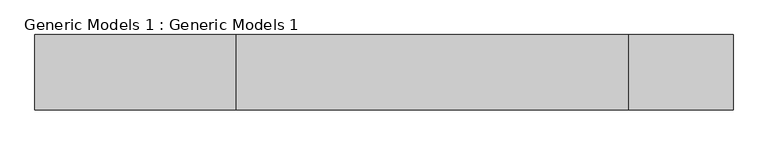
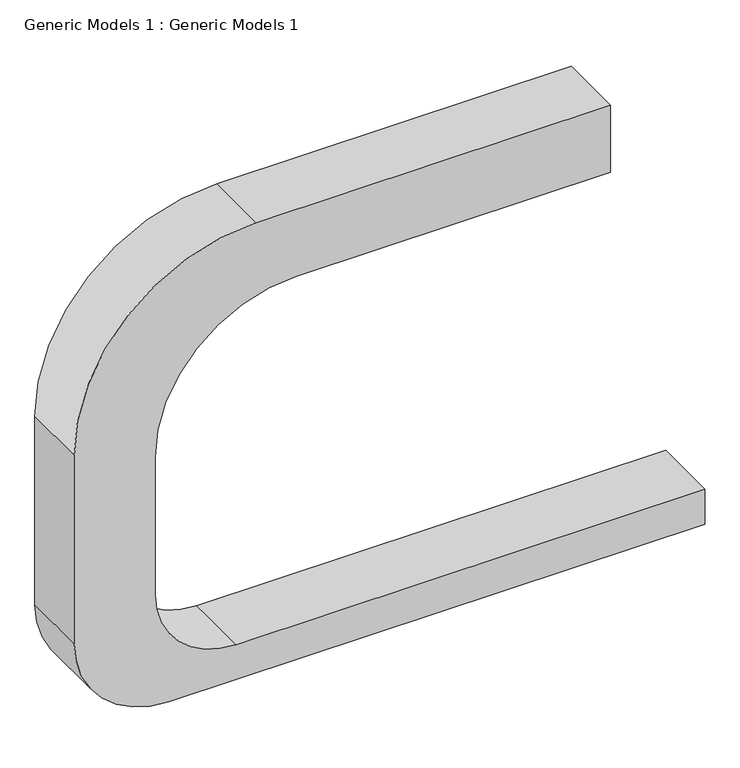
"""IFC4 building model written with IfcOpenShell, lengths in millimetres: proxy geometry, Generic Models 1 : Generic Models 1."""

from ifc_helpers import new_model, si_unit, point, frame, frame_2d, origin, place, context, project, spatial, polyline, circle_curve, trimmed, segment, composite_curve, outline, extrude, source, transform, mapped, element, save


def generic_models_1_generic_models_1_6508f6ba(model_context):
    return source(origin(), model_context, "Body", "SweptSolid", [
        extrude(outline(composite_curve([segment(polyline([(3600.4955814, -841.7906166), (3600.4955814, -7905.4681824)]), True, "CONTINUOUS"), segment(trimmed(circle_curve(frame_2d((4819.6955814, -7905.4681824)), 1219.2), [point((3600.4955814, -7905.4681824))], [point((4819.6955814, -9124.6681824))], True, "CARTESIAN"), True, "CONTINUOUS"), segment(polyline([(4819.6955814, -9124.6681824), (7010.4, -9124.6681824)]), True, "CONTINUOUS"), segment(trimmed(circle_curve(frame_2d((7010.4, -6991.0681824)), 2133.6), [point((7010.4, -9124.6681824))], [point((9144.0, -6991.0681824))], True, "CARTESIAN"), True, "CONTINUOUS"), segment(polyline([(9144.0, -6991.0681824), (9144.0, -2266.6681824), (10210.8, -2266.6681824), (10210.8, -7600.6681824)]), True, "CONTINUOUS"), segment(trimmed(circle_curve(frame_2d((7467.6, -7600.6681824)), 2743.2), [point((10210.8, -7600.6681824))], [point((7467.6, -10343.8681824))], False, "CARTESIAN"), True, "CONTINUOUS"), segment(polyline([(7467.6, -10343.8681824), (4470.4, -10343.8681824)]), True, "CONTINUOUS"), segment(trimmed(circle_curve(frame_2d((4470.4, -8921.4681824)), 1422.4), [point((4470.4, -10343.8681824))], [point((3048.0, -8921.4681824))], False, "CARTESIAN"), True, "CONTINUOUS"), segment(polyline([(3048.0, -8921.4681824), (3048.0, -841.7906166), (3600.4955814, -841.7906166)]), True, "CONTINUOUS")], self_intersect=False)), frame((0.0, -15615.172246, 0.0), z_axis=(0.0, 1.0, 0.0), x_axis=(0.0, 0.0, 1.0)), (0.0, 0.0, 1.0), 1024.261467),
    ])


if __name__ == "__main__":
    model = new_model("IFC4")
    model_context = context("Model", 3, world=origin())
    ifc_project = project(units=[si_unit("LENGTHUNIT", "METRE", prefix="MILLI")], contexts=[model_context])
    site = spatial("IfcSite", under=ifc_project)
    building = spatial("IfcBuilding", under=site)
    placement = place(None, origin())
    generic_models_1_generic_models_1_shape = generic_models_1_generic_models_1_6508f6ba(model_context)
    element("IfcBuildingElementProxy", 1, Name="Generic Models 1 : Generic Models 1", ObjectType="Generic Models 1 : Generic Models 1", at=placement, inside=building, context=model_context, shape_type="MappedRepresentation", body=[
        mapped(generic_models_1_generic_models_1_shape, transform((0.0, 0.0, 0.0), x_axis=(1.0, 0.0, 0.0), y_axis=(0.0, 1.0, 0.0), z_axis=(0.0, 0.0, 1.0))),
    ])
    save(model, "model.ifc")

# Revit data of these elements
# Element 1 (IfcBuildingElementProxy, "Generic Models 1 : Generic Models 1")
#   Materials on its faces: "Brick, Soldier Course", "Earth", "BLUE"
# Materials
#   "Brick, Soldier Course": class "Masonry", colour RGB 170 98 104, transparency 0, Description = "Common brick soldier coursed", Cost = 0
#   "Earth": class "Generic", colour RGB 97 75 62, transparency 0, Description = "Soil", Cost = 0
#   "BLUE": class "Generic", colour RGB 120 120 120, transparency 0, Cost = 0
